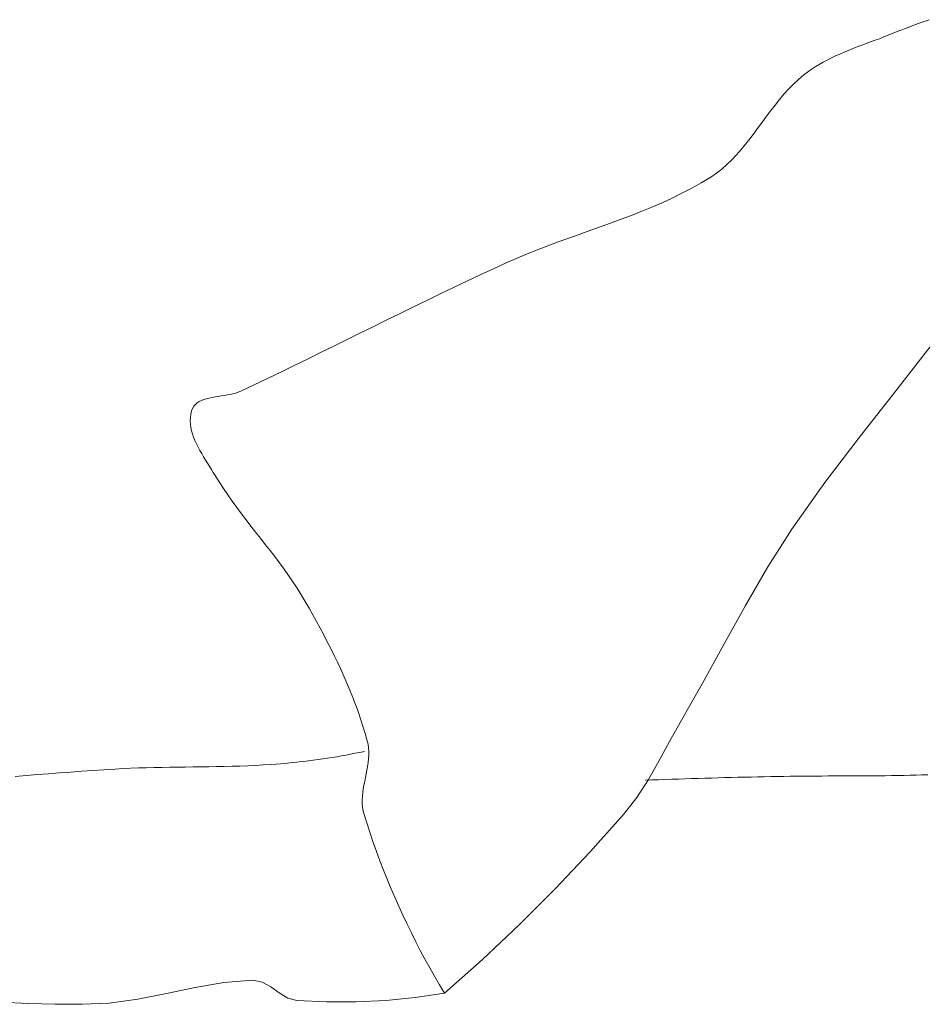
# Model space of a CAD drawing. Units: inches. Extents: x -15 to 423, y -713 to 71.
# Tile 12 of 24: x 308 to 333, y -342 to -315. Entities that reach past the tile are written whole.
import ezdxf

# ---------------------------------------------------------------- set-up
doc = ezdxf.new("R2010")
doc.units = ezdxf.units.IN
doc.header["$MEASUREMENT"] = 0
doc.layers.add('A-FURN', color=9, linetype='Continuous', lineweight=13)

# ---------------------------------------------------------------- blocks, each defined once
blk = doc.blocks.new('BED-DOUBLE')
for p, q in [((69.499, 27.193), (69.662, 27.255)), ((69.662, 27.255), (69.826, 27.318)), ((69.826, 27.318), (69.989, 27.379)), ((69.989, 27.379), (70.153, 27.439)), ((70.153, 27.439), (70.317, 27.499)), ((68.808, 26.923), (68.931, 26.969)), ((68.931, 26.969), (69.053, 27.016)), ((69.053, 27.016), (69.175, 27.064)), ((69.175, 27.064), (69.337, 27.129)), ((69.337, 27.129), (69.499, 27.193)), ((68.069, 26.642), (68.191, 26.69)), ((68.191, 26.69), (68.314, 26.738)), ((68.314, 26.738), (68.438, 26.784)), ((68.438, 26.784), (68.561, 26.831)), ((68.561, 26.831), (68.685, 26.877)), ((68.685, 26.877), (68.808, 26.923)), ((67.472, 26.373), (67.589, 26.431)), ((67.589, 26.431), (67.707, 26.487)), ((67.707, 26.487), (67.826, 26.54)), ((67.826, 26.54), (67.947, 26.592)), ((67.947, 26.592), (68.069, 26.642)), ((67.025, 26.11), (67.133, 26.181)), ((67.133, 26.181), (67.244, 26.248)), ((67.244, 26.248), (67.357, 26.312)), ((67.357, 26.312), (67.472, 26.373)), ((66.668, 25.831), (66.815, 25.956)), ((66.815, 25.956), (66.919, 26.035)), ((66.919, 26.035), (67.025, 26.11)), ((66.394, 25.561), (66.528, 25.699)), ((66.528, 25.699), (66.668, 25.831)), ((66.139, 25.268), (66.264, 25.417)), ((66.264, 25.417), (66.394, 25.561)), ((65.898, 24.96), (66.017, 25.115)), ((66.017, 25.115), (66.139, 25.268)), ((65.664, 24.644), (65.781, 24.803)), ((65.781, 24.803), (65.898, 24.96)), ((65.432, 24.329), (65.548, 24.486)), ((65.548, 24.486), (65.664, 24.644)), ((65.313, 24.173), (65.432, 24.329)), ((65.07, 23.871), (65.193, 24.02)), ((65.193, 24.02), (65.313, 24.173)), ((64.81, 23.587), (64.942, 23.726)), ((64.942, 23.726), (65.07, 23.871)), ((64.529, 23.329), (64.673, 23.454)), ((64.673, 23.454), (64.81, 23.587)), ((63.956, 22.943), (64.219, 23.104)), ((64.219, 23.104), (64.378, 23.211)), ((64.378, 23.211), (64.529, 23.329)), ((63.688, 22.792), (63.956, 22.943)), ((63.139, 22.515), (63.415, 22.65)), ((63.415, 22.65), (63.688, 22.792)), ((62.576, 22.264), (62.859, 22.386)), ((62.859, 22.386), (63.139, 22.515)), ((61.713, 21.924), (62.003, 22.034)), ((62.003, 22.034), (62.291, 22.147)), ((62.291, 22.147), (62.576, 22.264)), ((61.13, 21.712), (61.422, 21.817)), ((61.422, 21.817), (61.713, 21.924)), ((60.252, 21.4), (60.545, 21.504)), ((60.545, 21.504), (60.838, 21.608)), ((60.838, 21.608), (61.13, 21.712)), ((59.38, 21.075), (59.67, 21.186)), ((59.67, 21.186), (59.96, 21.294)), ((59.96, 21.294), (60.252, 21.4)), ((58.808, 20.841), (59.093, 20.96)), ((59.093, 20.96), (59.38, 21.075)), ((58.15, 20.544), (58.525, 20.716)), ((58.525, 20.716), (58.808, 20.841)), ((57.402, 20.194), (57.776, 20.37)), ((57.776, 20.37), (58.15, 20.544)), ((57.029, 20.017), (57.402, 20.194)), ((56.286, 19.659), (56.657, 19.838)), ((56.657, 19.838), (57.029, 20.017)), ((55.915, 19.478), (56.286, 19.659)), ((55.173, 19.115), (55.544, 19.297)), ((55.544, 19.297), (55.915, 19.478)), ((54.803, 18.932), (55.173, 19.115)), ((54.063, 18.567), (54.433, 18.75)), ((54.433, 18.75), (54.803, 18.932)), ((53.692, 18.384), (54.063, 18.567)), ((52.951, 18.021), (53.322, 18.202)), ((53.322, 18.202), (53.692, 18.384)), ((70.336, 18.355), (69.362, 17.092)), ((52.58, 17.84), (52.951, 18.021)), ((51.837, 17.48), (52.209, 17.659)), ((52.209, 17.659), (52.58, 17.84)), ((51.465, 17.303), (51.837, 17.48)), ((50.791, 17.034), (50.871, 17.052)), ((50.871, 17.052), (50.948, 17.073)), ((50.948, 17.073), (51.022, 17.097)), ((51.022, 17.097), (51.091, 17.126)), ((51.091, 17.126), (51.465, 17.303)), ((69.362, 17.092), (68.377, 15.838)), ((49.822, 16.751), (49.873, 16.795)), ((49.873, 16.795), (49.93, 16.832)), ((49.93, 16.832), (49.993, 16.864)), ((49.993, 16.864), (50.062, 16.891)), ((50.062, 16.891), (50.135, 16.914)), ((50.135, 16.914), (50.211, 16.933)), ((50.211, 16.933), (50.291, 16.95)), ((50.291, 16.95), (50.373, 16.965)), ((50.373, 16.965), (50.456, 16.978)), ((50.456, 16.978), (50.541, 16.991)), ((50.541, 16.991), (50.625, 17.004)), ((50.625, 17.004), (50.709, 17.018)), ((50.709, 17.018), (50.791, 17.034)), ((49.695, 16.485), (49.718, 16.577)), ((49.718, 16.577), (49.744, 16.643)), ((49.744, 16.643), (49.779, 16.701)), ((49.779, 16.701), (49.822, 16.751)), ((49.678, 16.3), (49.682, 16.392)), ((49.683, 16.207), (49.678, 16.3)), ((49.682, 16.392), (49.695, 16.485)), ((49.695, 16.114), (49.683, 16.207)), ((49.715, 16.021), (49.695, 16.114)), ((49.741, 15.928), (49.715, 16.021)), ((49.773, 15.836), (49.741, 15.928)), ((49.811, 15.743), (49.773, 15.836)), ((49.853, 15.651), (49.811, 15.743)), ((68.377, 15.838), (67.408, 14.572)), ((49.898, 15.56), (49.853, 15.651)), ((49.947, 15.469), (49.898, 15.56)), ((49.999, 15.379), (49.947, 15.469)), ((50.052, 15.289), (49.999, 15.379)), ((50.106, 15.2), (50.052, 15.289)), ((50.161, 15.113), (50.106, 15.2)), ((50.216, 15.026), (50.161, 15.113)), ((50.27, 14.94), (50.216, 15.026)), ((50.323, 14.856), (50.27, 14.94)), ((50.373, 14.773), (50.323, 14.856)), ((50.486, 14.588), (50.373, 14.773)), ((50.604, 14.407), (50.486, 14.588)), ((50.725, 14.228), (50.604, 14.407)), ((67.408, 14.572), (66.487, 13.273)), ((50.85, 14.051), (50.725, 14.228)), ((50.978, 13.876), (50.85, 14.051)), ((51.107, 13.702), (50.978, 13.876)), ((51.239, 13.53), (51.107, 13.702)), ((51.372, 13.358), (51.239, 13.53)), ((51.506, 13.188), (51.372, 13.358)), ((66.487, 13.273), (65.818, 12.219)), ((51.64, 13.017), (51.506, 13.188)), ((51.775, 12.846), (51.64, 13.017)), ((51.908, 12.675), (51.775, 12.846)), ((52.04, 12.503), (51.908, 12.675)), ((52.171, 12.33), (52.04, 12.503)), ((52.299, 12.156), (52.171, 12.33)), ((52.425, 11.98), (52.299, 12.156)), ((65.818, 12.219), (65.191, 11.14)), ((52.548, 11.802), (52.425, 11.98)), ((52.667, 11.621), (52.548, 11.802)), ((52.782, 11.438), (52.667, 11.621)), ((52.892, 11.252), (52.782, 11.438)), ((52.997, 11.067), (52.892, 11.252)), ((53.102, 10.881), (52.997, 11.067)), ((65.191, 11.14), (64.585, 10.047)), ((53.205, 10.694), (53.102, 10.881)), ((53.307, 10.506), (53.205, 10.694)), ((53.407, 10.317), (53.307, 10.506)), ((53.506, 10.127), (53.407, 10.317)), ((53.603, 9.937), (53.506, 10.127)), ((53.698, 9.745), (53.603, 9.937)), ((64.585, 10.047), (63.982, 8.952)), ((53.791, 9.552), (53.698, 9.745)), ((53.881, 9.358), (53.791, 9.552)), ((53.969, 9.163), (53.881, 9.358)), ((54.054, 8.968), (53.969, 9.163)), ((54.137, 8.771), (54.054, 8.968)), ((63.982, 8.952), (63.363, 7.868)), ((54.217, 8.573), (54.137, 8.771)), ((54.293, 8.374), (54.217, 8.573)), ((54.366, 8.174), (54.293, 8.374)), ((54.436, 7.972), (54.366, 8.174)), ((54.503, 7.77), (54.436, 7.972)), ((54.565, 7.566), (54.503, 7.77)), ((63.363, 7.868), (63.066, 7.342)), ((54.624, 7.362), (54.565, 7.566)), ((54.647, 7.262), (54.624, 7.362)), ((54.66, 7.161), (54.647, 7.262)), ((54.666, 7.059), (54.66, 7.161)), ((63.066, 7.342), (62.776, 6.809)), ((53.64, 6.895), (53.51, 6.874)), ((53.77, 6.916), (53.64, 6.895)), ((53.901, 6.938), (53.77, 6.916)), ((54.031, 6.961), (53.901, 6.938)), ((54.16, 6.985), (54.031, 6.961)), ((54.29, 7.01), (54.16, 6.985)), ((54.419, 7.036), (54.29, 7.01)), ((54.549, 7.062), (54.419, 7.036)), ((54.659, 6.853), (54.666, 6.957)), ((54.666, 6.957), (54.666, 7.059)), ((48.232, 6.602), (48.014, 6.593)), ((48.45, 6.608), (48.232, 6.602)), ((48.668, 6.614), (48.45, 6.608)), ((48.886, 6.618), (48.668, 6.614)), ((49.104, 6.622), (48.886, 6.618)), ((49.322, 6.624), (49.104, 6.622)), ((49.54, 6.627), (49.322, 6.624)), ((49.758, 6.629), (49.54, 6.627)), ((49.976, 6.632), (49.758, 6.629)), ((50.194, 6.635), (49.976, 6.632)), ((50.412, 6.638), (50.194, 6.635)), ((50.63, 6.642), (50.412, 6.638)), ((50.847, 6.648), (50.63, 6.642)), ((51.065, 6.654), (50.847, 6.648)), ((51.283, 6.662), (51.065, 6.654)), ((51.501, 6.672), (51.283, 6.662)), ((51.718, 6.684), (51.501, 6.672)), ((51.936, 6.698), (51.718, 6.684)), ((52.067, 6.708), (51.936, 6.698)), ((52.199, 6.719), (52.067, 6.708)), ((52.33, 6.73), (52.199, 6.719)), ((52.462, 6.743), (52.33, 6.73)), ((52.593, 6.756), (52.462, 6.743)), ((52.724, 6.77), (52.593, 6.756)), ((52.855, 6.785), (52.724, 6.77)), ((52.986, 6.801), (52.855, 6.785)), ((53.117, 6.818), (52.986, 6.801)), ((53.248, 6.836), (53.117, 6.818)), ((53.379, 6.855), (53.248, 6.836)), ((53.51, 6.874), (53.379, 6.855)), ((54.614, 6.54), (54.632, 6.645)), ((54.632, 6.645), (54.647, 6.749)), ((54.647, 6.749), (54.659, 6.853)), ((62.776, 6.809), (62.478, 6.283)), ((45.1, 6.391), (44.791, 6.365)), ((45.41, 6.416), (45.1, 6.391)), ((45.72, 6.441), (45.41, 6.416)), ((46.029, 6.465), (45.72, 6.441)), ((46.339, 6.488), (46.029, 6.465)), ((46.649, 6.51), (46.339, 6.488)), ((46.959, 6.532), (46.649, 6.51)), ((47.269, 6.552), (46.959, 6.532)), ((47.579, 6.571), (47.269, 6.552)), ((47.797, 6.583), (47.579, 6.571)), ((48.014, 6.593), (47.797, 6.583)), ((54.552, 6.226), (54.573, 6.331)), ((54.573, 6.331), (54.594, 6.436)), ((54.594, 6.436), (54.614, 6.54)), ((64.238, 6.32), (64.423, 6.325)), ((64.423, 6.325), (64.607, 6.33)), ((64.607, 6.33), (64.792, 6.335)), ((64.792, 6.335), (64.977, 6.34)), ((64.977, 6.34), (65.162, 6.344)), ((65.162, 6.344), (65.346, 6.348)), ((65.346, 6.348), (65.531, 6.352)), ((65.531, 6.352), (65.716, 6.356)), ((65.716, 6.356), (65.901, 6.36)), ((65.901, 6.36), (66.086, 6.364)), ((66.086, 6.364), (66.263, 6.367)), ((66.263, 6.367), (66.439, 6.369)), ((66.439, 6.369), (66.616, 6.371)), ((66.616, 6.371), (66.793, 6.373)), ((66.793, 6.373), (66.97, 6.374)), ((66.97, 6.374), (67.147, 6.375)), ((67.147, 6.375), (67.324, 6.376)), ((67.324, 6.376), (67.501, 6.377)), ((67.501, 6.377), (67.678, 6.377)), ((67.678, 6.377), (67.855, 6.378)), ((67.855, 6.378), (68.031, 6.378)), ((68.031, 6.378), (68.208, 6.379)), ((68.208, 6.379), (68.385, 6.38)), ((68.385, 6.38), (68.562, 6.381)), ((68.562, 6.381), (68.739, 6.382)), ((68.739, 6.382), (68.916, 6.383)), ((68.916, 6.383), (69.093, 6.385)), ((69.093, 6.385), (69.27, 6.388)), ((69.27, 6.388), (69.447, 6.391)), ((69.447, 6.391), (69.624, 6.394)), ((69.624, 6.394), (69.789, 6.398)), ((69.789, 6.398), (69.954, 6.401)), ((69.954, 6.401), (70.12, 6.405)), ((70.12, 6.405), (70.285, 6.41)), ((54.514, 6.017), (54.532, 6.121)), ((54.532, 6.121), (54.552, 6.226)), ((62.478, 6.283), (62.152, 5.777)), ((62.39, 6.259), (62.575, 6.266)), ((62.575, 6.266), (62.76, 6.273)), ((62.76, 6.273), (62.945, 6.279)), ((62.945, 6.279), (63.129, 6.286)), ((63.129, 6.286), (63.314, 6.292)), ((63.314, 6.292), (63.499, 6.298)), ((63.499, 6.298), (63.684, 6.304)), ((63.684, 6.304), (63.868, 6.309)), ((63.868, 6.309), (64.053, 6.315)), ((64.053, 6.315), (64.238, 6.32)), ((54.485, 5.706), (54.49, 5.809)), ((54.49, 5.809), (54.5, 5.913)), ((54.5, 5.913), (54.514, 6.017)), ((62.152, 5.777), (61.784, 5.302)), ((54.485, 5.604), (54.485, 5.706)), ((54.494, 5.503), (54.485, 5.604)), ((54.51, 5.403), (54.494, 5.503)), ((54.535, 5.304), (54.51, 5.403)), ((54.617, 5.043), (54.535, 5.304)), ((61.784, 5.302), (60.841, 4.249)), ((54.702, 4.782), (54.617, 5.043)), ((54.791, 4.523), (54.702, 4.782)), ((54.883, 4.264), (54.791, 4.523)), ((54.978, 4.007), (54.883, 4.264)), ((60.841, 4.249), (59.869, 3.223)), ((55.077, 3.75), (54.978, 4.007)), ((55.178, 3.495), (55.077, 3.75)), ((55.283, 3.241), (55.178, 3.495)), ((55.392, 2.989), (55.283, 3.241)), ((59.869, 3.223), (58.868, 2.224)), ((55.503, 2.738), (55.392, 2.989)), ((55.617, 2.488), (55.503, 2.738)), ((55.735, 2.239), (55.617, 2.488)), ((55.856, 1.992), (55.735, 2.239)), ((58.868, 2.224), (57.839, 1.253)), ((55.979, 1.747), (55.856, 1.992)), ((56.106, 1.504), (55.979, 1.747)), ((56.236, 1.262), (56.106, 1.504)), ((56.369, 1.022), (56.236, 1.262)), ((57.839, 1.253), (56.785, 0.313)), ((56.504, 0.783), (56.369, 1.022)), ((50.62, 0.613), (49.818, 0.473)), ((51.429, 0.676), (50.62, 0.613)), ((51.688, 0.622), (51.429, 0.676)), ((51.928, 0.485), (51.688, 0.622)), ((56.643, 0.547), (56.504, 0.783)), ((49.019, 0.3), (48.217, 0.14)), ((49.818, 0.473), (49.019, 0.3)), ((52.162, 0.319), (51.928, 0.485)), ((52.401, 0.174), (52.162, 0.319)), ((56.785, 0.313), (55.966, 0.192)), ((56.785, 0.313), (56.643, 0.547)), ((45.149, 0.023), (44.395, 0.056)), ((45.904, 0), (45.149, 0.023)), ((46.658, 0), (45.904, 0)), ((47.41, 0.036), (46.658, 0)), ((48.217, 0.14), (47.41, 0.036)), ((52.659, 0.102), (52.401, 0.174)), ((53.485, 0.066), (52.659, 0.102)), ((54.314, 0.069), (53.485, 0.066)), ((55.142, 0.111), (54.314, 0.069)), ((55.966, 0.192), (55.142, 0.111))]:
    blk.add_line(p, q)

msp = doc.modelspace()

# ---------------------------------------------------------------- block references
at = {"layer": 'A-FURN'}
msp.add_blockref('BED-DOUBLE', (262.678, -342.175), dxfattribs=at)

doc.saveas('drawing.dxf')
